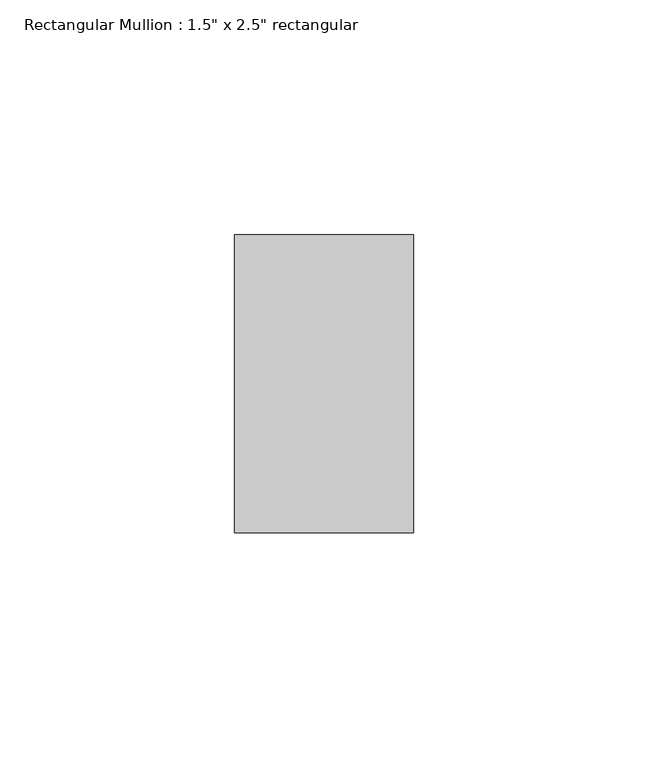
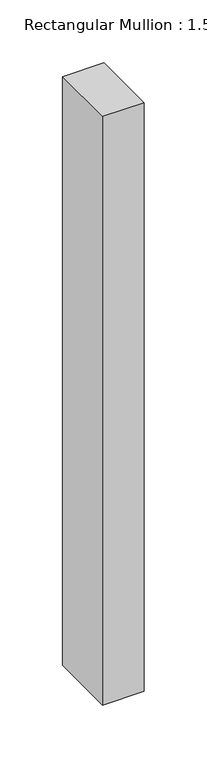
"""IFC4 building model written with IfcOpenShell, lengths in millimetres: member geometry."""

from ifc_helpers import new_model, si_unit, frame, origin, place, context, project, spatial, polyline, outline, extrude, source, transform, mapped, element, save


def member_a67f877f(model_context):
    return source(origin(), model_context, "Body", "SweptSolid", [
        extrude(outline(polyline([(0.0, 31.75), (0.0, -31.75), (-38.1, -31.75), (-38.1, 31.75), (0.0, 31.75)])), frame((0.0, 0.0, -571.5), z_axis=(0.0, 0.0, 1.0), x_axis=(1.0, 0.0, 0.0)), (0.0, 0.0, 1.0), 571.5),
    ])


if __name__ == "__main__":
    model = new_model("IFC4")
    model_context = context("Model", 3, world=origin())
    ifc_project = project(units=[si_unit("LENGTHUNIT", "METRE", prefix="MILLI")], contexts=[model_context])
    site = spatial("IfcSite", under=ifc_project)
    building = spatial("IfcBuilding", under=site)
    placement = place(None, origin())
    member_shape = member_a67f877f(model_context)
    element("IfcMember", 1, ObjectType="Rectangular Mullion : 1.5\" x 2.5\" rectangular", at=placement, inside=building, context=model_context, shape_type="MappedRepresentation", body=[
        mapped(member_shape, transform((0.0, 0.0, 0.0), x_axis=(1.0, 0.0, 0.0), y_axis=(0.0, 1.0, 0.0), z_axis=(0.0, 0.0, 1.0))),
    ])
    save(model, "model.ifc")

# Revit data of these elements
# Type "Rectangular Mullion : 1.5\" x 2.5\" rectangular"
#   built-in parameter 1007304 = 0.208333 (stored number, unit not read)
#   built-in parameter 1007301 = 0.0625 (stored number, unit not read)
#   built-in parameter 1007300 = 0.0625 (stored number, unit not read)
